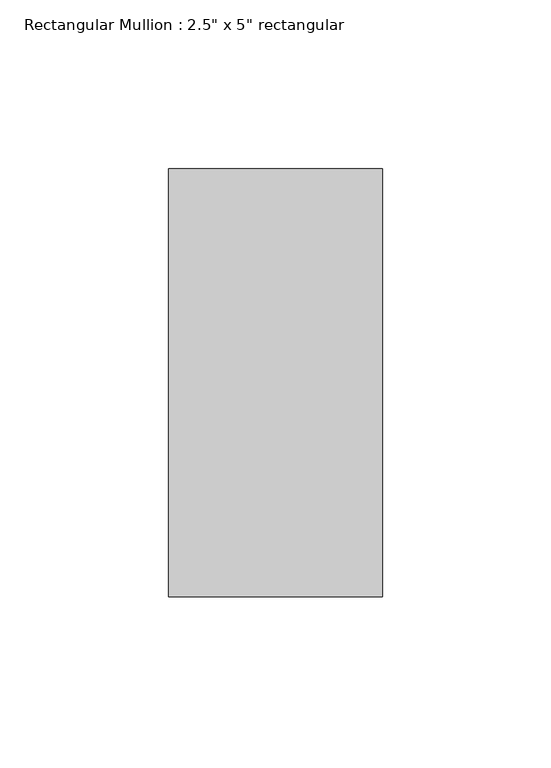
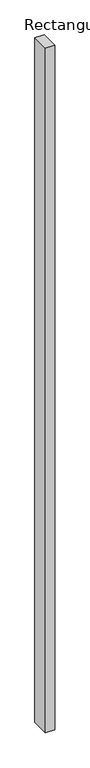
"""IFC4 building model written with IfcOpenShell, lengths in millimetres: member geometry."""

from ifc_helpers import new_model, si_unit, frame, origin, place, context, project, spatial, polyline, outline, extrude, source, transform, mapped, element, save


def member_94311e20(model_context):
    return source(origin(), model_context, "Body", "SweptSolid", [
        extrude(outline(polyline([(0.0, 63.5), (0.0, -63.5), (-63.5, -63.5), (-63.5, 63.5), (0.0, 63.5)])), frame((0.0, 0.0, -5029.2), z_axis=(0.0, 0.0, 1.0), x_axis=(1.0, 0.0, 0.0)), (0.0, 0.0, 1.0), 5029.2),
    ])


if __name__ == "__main__":
    model = new_model("IFC4")
    model_context = context("Model", 3, world=origin())
    ifc_project = project(units=[si_unit("LENGTHUNIT", "METRE", prefix="MILLI")], contexts=[model_context])
    site = spatial("IfcSite", under=ifc_project)
    building = spatial("IfcBuilding", under=site)
    placement = place(None, origin())
    member_shape = member_94311e20(model_context)
    element("IfcMember", 1, ObjectType="Rectangular Mullion : 2.5\" x 5\" rectangular", at=placement, inside=building, context=model_context, shape_type="MappedRepresentation", body=[
        mapped(member_shape, transform((0.0, 0.0, 0.0), x_axis=(1.0, 0.0, 0.0), y_axis=(0.0, 1.0, 0.0), z_axis=(0.0, 0.0, 1.0))),
    ])
    save(model, "model.ifc")

# Revit data of these elements
# Type "Rectangular Mullion : 2.5\" x 5\" rectangular"
#   built-in parameter 1007304 = 0.416667 (stored number, unit not read)
#   built-in parameter 1007301 = 0.104167 (stored number, unit not read)
#   built-in parameter 1007300 = 0.104167 (stored number, unit not read)
# Element 1 (IfcMember, "Rectangular Mullion : 2.5\" x 5\" rectangular")
#   Materials on its faces: "Aluminum"
# Materials
#   "Aluminum": class "Metal", colour RGB 247 247 247, transparency 0, Description = "Aluminum 6061", Cost = 0
